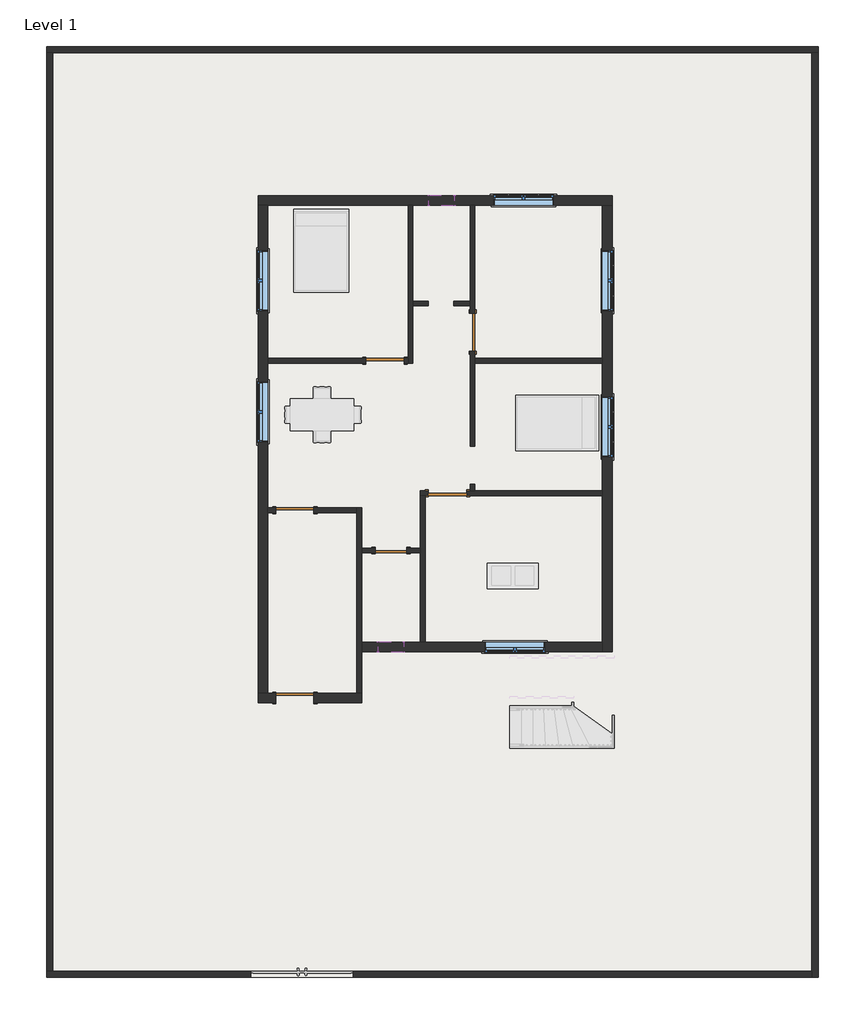
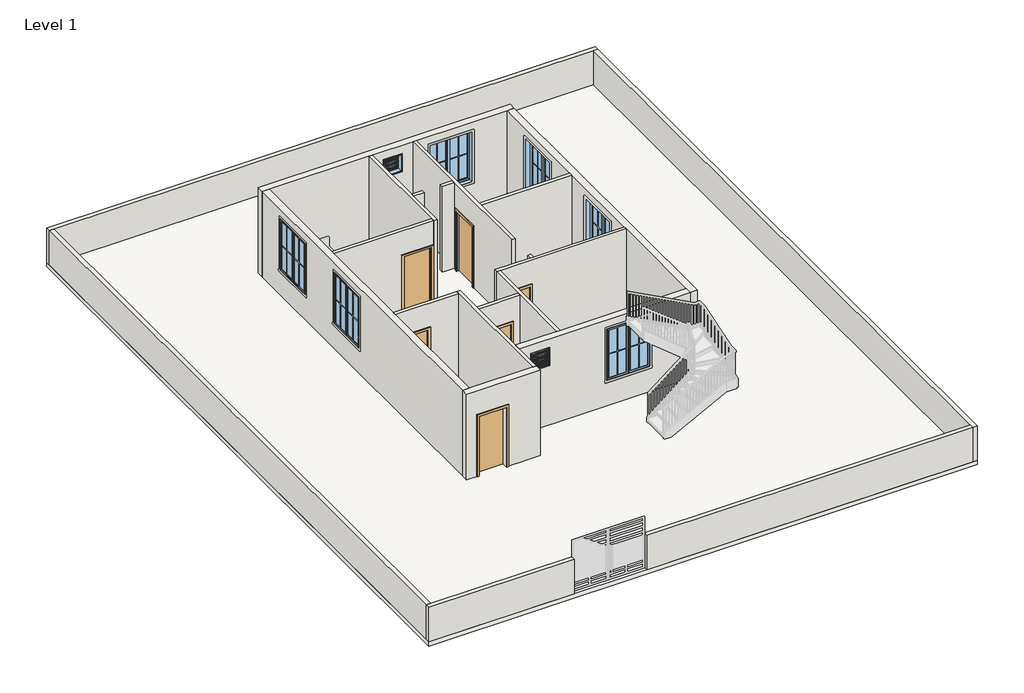
# One storey, part 1 of 3: 22 walls, 8 windows, 6 doors, 1 slab.
"""IFC4 building model written with IfcOpenShell, lengths in millimetres."""

from ifc_helpers import new_model, si_unit, frame, origin, origin_with_axes, place, context, project, spatial, polyline, outline, extrude, faceted_brep, transform, mapped, element, save
from components import door_214872d5, single_flush_door_3_e5f9f3c4, single_flush_door_3_305aa2a5, single_flush_door_3_a90ba1ad, window_9ac97e1a, window_f2d8fef0

model = new_model("IFC4")

# Units and contexts
model_context = context("Model", 3, world=origin())
ifc_project = project(units=[si_unit("LENGTHUNIT", "METRE", prefix="MILLI")], contexts=[model_context])

# Site, building, storey
site = spatial("IfcSite", under=ifc_project)
building = spatial("IfcBuilding", under=site)
storey = spatial("IfcBuildingStorey", under=building, Name="Level 1", Elevation=0.0)

# Doors
placement = place(None, origin())
door_shape = door_214872d5(model_context)
element("IfcDoor", 1, ObjectType="Single-Flush : DOOR 2'6\"", at=placement, inside=storey, context=model_context, shape_type="MappedRepresentation", body=[
    mapped(door_shape, transform((-2309.3144966, -2885.2590409, 0.0), x_axis=(-1.0, 0.0, 0.0), y_axis=(0.0, -1.0, 0.0), z_axis=(0.0, 0.0, 1.0))),
])
single_flush_door_3_shape = single_flush_door_3_e5f9f3c4(model_context)
element("IfcDoor", 2, ObjectType="Single-Flush : DOOR 3'", at=placement, inside=storey, context=model_context, shape_type="MappedRepresentation", body=[
    mapped(single_flush_door_3_shape, transform((-2455.3644966, 1648.6409591, 0.0), x_axis=(1.0, 0.0, 0.0), y_axis=(0.0, 1.0, 0.0), z_axis=(0.0, 0.0, 1.0))),
])
element("IfcDoor", 3, ObjectType="Single-Flush : DOOR 3'", at=placement, inside=storey, context=model_context, shape_type="MappedRepresentation", body=[
    mapped(single_flush_door_3_shape, transform((-359.8644966, 2334.4409591, 0.0), x_axis=(0.0, -1.0, 0.0), y_axis=(1.0, 0.0, 0.0), z_axis=(0.0, 0.0, 1.0))),
])
element("IfcDoor", 4, ObjectType="Single-Flush : DOOR 3'", at=placement, inside=storey, context=model_context, shape_type="MappedRepresentation", body=[
    mapped(single_flush_door_3_shape, transform((-956.7644966, -1513.6590409, 0.0), x_axis=(-1.0, 0.0, 0.0), y_axis=(0.0, -1.0, 0.0), z_axis=(0.0, 0.0, 1.0))),
])
single_flush_door_3_2_shape = single_flush_door_3_305aa2a5(model_context)
element("IfcDoor", 5, ObjectType="Single-Flush : DOOR 3'", at=placement, inside=storey, context=model_context, shape_type="MappedRepresentation", body=[
    mapped(single_flush_door_3_2_shape, transform((-4608.0144966, -1920.0590409, 0.0), x_axis=(-1.0, 0.0, 0.0), y_axis=(0.0, -1.0, 0.0), z_axis=(0.0, 0.0, 1.0))),
])
single_flush_door_3_3_shape = single_flush_door_3_a90ba1ad(model_context)
element("IfcDoor", 6, ObjectType="Single-Flush : DOOR 3'", at=placement, inside=storey, context=model_context, shape_type="MappedRepresentation", body=[
    mapped(single_flush_door_3_3_shape, transform((-4608.0144966, -6409.5090409, 0.0), x_axis=(-1.0, 0.0, 0.0), y_axis=(0.0, -1.0, 0.0), z_axis=(0.0, 0.0, 1.0))),
])

# Slab
element("IfcSlab", 7, ObjectType="FLOOR 6\"", at=placement, inside=storey, context=model_context, shape_type="SweptSolid", body=[
    extrude(outline(polyline([(7897.8751323, 9160.4523528), (7897.8751323, -13089.9476472), (-10542.5248677, -13089.9476472), (-10542.5248677, 9160.4523528), (7897.8751323, 9160.4523528)])), frame((0.0, 0.0, -152.4), z_axis=(0.0, 0.0, 1.0), x_axis=(1.0, 0.0, 0.0)), (0.0, 0.0, 1.0), 152.4),
])

# Walls
element("IfcWall", 8, ObjectType="CMD 6\"", at=placement, inside=storey, context=model_context, shape_type="Brep", body=[
    faceted_brep([(-10542.5248677, 9008.0523528, 0.0), (-10390.1248677, 9008.0523528, 0.0), (7745.4751323, 9008.0523528, 0.0), (7897.8751323, 9008.0523528, 0.0), (7897.8751323, 9008.0523528, 1219.2), (7745.4751323, 9008.0523528, 1219.2), (-10390.1248677, 9008.0523528, 1219.2), (-10542.5248677, 9008.0523528, 1219.2), (-10542.5248677, 9160.4523528, 0.0), (-10542.5248677, 9160.4523528, 1219.2), (7897.8751323, 9160.4523528, 1219.2), (7897.8751323, 9160.4523528, 0.0)], [[[0, 1, 2, 3, 4, 5, 6, 7]], [[8, 9, 10, 11]], [[3, 2, 1, 0, 8, 11]], [[7, 6, 5, 4, 10, 9]], [[4, 3, 11, 10]], [[0, 7, 9, 8]]]),
])
element("IfcWall", 9, ObjectType="CMD 6\"", at=placement, inside=storey, context=model_context, shape_type="Brep", body=[
    faceted_brep([(7745.4751323, 9008.0523528, 0.0), (7745.4751323, -12937.5476472, 0.0), (7745.4751323, -13089.9476472, 0.0), (7745.4751323, -13089.9476472, 1219.2), (7745.4751323, -12937.5476472, 1219.2), (7745.4751323, 9008.0523528, 1219.2), (7897.8751323, 9008.0523528, 0.0), (7897.8751323, 9008.0523528, 1219.2), (7897.8751323, -13089.9476472, 1219.2), (7897.8751323, -13089.9476472, 0.0)], [[[0, 1, 2, 3, 4, 5]], [[6, 7, 8, 9]], [[2, 1, 0, 6, 9]], [[5, 4, 3, 8, 7]], [[0, 5, 7, 6]], [[3, 2, 9, 8]]]),
])
element("IfcWall", 10, ObjectType="CMD 6\"", at=placement, inside=storey, context=model_context, shape_type="SweptSolid", body=[
    extrude(outline(polyline([(-3217.3644966, -12937.5476472), (7745.4751323, -12937.5476472), (7745.4751323, -13089.9476472), (-3217.3644966, -13089.9476472), (-3217.3644966, -12937.5476472)])), origin_with_axes(), (0.0, 0.0, 1.0), 1219.2),
])
element("IfcWall", 11, ObjectType="CMD 6\"", at=placement, inside=storey, context=model_context, shape_type="SweptSolid", body=[
    extrude(outline(polyline([(-10390.1248677, 9008.0523528), (-10390.1248677, -12937.5476472), (-10542.5248677, -12937.5476472), (-10542.5248677, 9008.0523528), (-10390.1248677, 9008.0523528)])), origin_with_axes(), (0.0, 0.0, 1.0), 1219.2),
])
element("IfcWall", 12, ObjectType="CMD 6\"", at=placement, inside=storey, context=model_context, shape_type="Brep", body=[
    faceted_brep([(-5655.7644966, -12937.5476472, 0.0), (-10390.1248677, -12937.5476472, 0.0), (-10542.5248677, -12937.5476472, 0.0), (-10542.5248677, -12937.5476472, 1219.2), (-10390.1248677, -12937.5476472, 1219.2), (-5655.7644966, -12937.5476472, 1219.2), (-5655.7644966, -13089.9476472, 0.0), (-5655.7644966, -13089.9476472, 1219.2), (-10542.5248677, -13089.9476472, 1219.2), (-10542.5248677, -13089.9476472, 0.0)], [[[0, 1, 2, 3, 4, 5]], [[6, 7, 8, 9]], [[2, 1, 0, 6, 9]], [[5, 4, 3, 8, 7]], [[0, 5, 7, 6]], [[3, 2, 9, 8]]]),
])
element("IfcWall", 13, ObjectType="WALL 4.5\"", at=placement, inside=storey, context=model_context, shape_type="Brep", body=[
    faceted_brep([(-1902.9144966, 5363.3909591, 0.0), (-1902.9144966, 1705.7909591, 0.0), (-1902.9144966, 1591.4909591, 0.0), (-1902.9144966, 1591.4909591, 3048.0), (-1902.9144966, 1705.7909591, 3048.0), (-1902.9144966, 5363.3909591, 3048.0), (-1788.6144966, 5363.3909591, 0.0), (-1788.6144966, 5363.3909591, 3048.0), (-1788.6144966, 3077.3909591, 3048.0), (-1788.6144966, 2963.0909591, 3048.0), (-1788.6144966, 1591.4909591, 3048.0), (-1788.6144966, 1591.4909591, 0.0), (-1788.6144966, 2963.0909591, 0.0), (-1788.6144966, 3077.3909591, 0.0)], [[[0, 1, 2, 3, 4, 5]], [[6, 7, 8, 9, 10, 11, 12, 13]], [[2, 1, 0, 6, 13, 12, 11]], [[0, 5, 7, 6]], [[3, 2, 11, 10]], [[5, 4, 3, 10, 9, 8, 7]]]),
])
element("IfcWall", 14, ObjectType="WALL 4.5\"", at=placement, inside=storey, context=model_context, shape_type="SweptSolid", body=[
    extrude(outline(polyline([(2133.6, -1998.1644966), (0.0, -1998.1644966), (0.0, -1902.9144966), (3048.0, -1902.9144966), (3048.0, -5255.7144966), (0.0, -5255.7144966), (0.0, -2912.5644966), (2133.6, -2912.5644966), (2133.6, -1998.1644966)])), frame((0.0, 1591.4909591, 0.0), z_axis=(0.0, 1.0, 0.0), x_axis=(0.0, 0.0, 1.0)), (0.0, 0.0, 1.0), 114.3),
])
element("IfcWall", 15, ObjectType="WALL 4.5\"", at=placement, inside=storey, context=model_context, shape_type="Brep", body=[
    faceted_brep([(-417.0144966, 1877.2409591, 2133.6), (-417.0144966, 1877.2409591, 0.0), (-417.0144966, -389.7090409, 0.0), (-417.0144966, -389.7090409, 3048.0), (-417.0144966, 2963.0909591, 3048.0), (-417.0144966, 3077.3909591, 3048.0), (-417.0144966, 5363.3909591, 3048.0), (-417.0144966, 5363.3909591, 0.0), (-417.0144966, 3077.3909591, 0.0), (-417.0144966, 2963.0909591, 0.0), (-417.0144966, 2791.6409591, 0.0), (-417.0144966, 2791.6409591, 2133.6), (-302.7144966, -389.7090409, 0.0), (-302.7144966, 1591.4909591, 0.0), (-302.7144966, 1705.7909591, 0.0), (-302.7144966, 1877.2409591, 0.0), (-302.7144966, 1877.2409591, 2133.6), (-302.7144966, 2791.6409591, 2133.6), (-302.7144966, 2791.6409591, 0.0), (-302.7144966, 5363.3909591, 0.0), (-302.7144966, 5363.3909591, 3048.0), (-302.7144966, 1705.7909591, 3048.0), (-302.7144966, 1591.4909591, 3048.0), (-302.7144966, -389.7090409, 3048.0)], [[[0, 1, 2, 3, 4, 5, 6, 7, 8, 9, 10, 11]], [[12, 13, 14, 15, 16, 17, 18, 19, 20, 21, 22, 23]], [[2, 1, 15, 14, 13, 12]], [[10, 9, 8, 7, 19, 18]], [[3, 2, 12, 23]], [[7, 6, 20, 19]], [[16, 15, 1, 0]], [[17, 16, 0, 11]], [[18, 17, 11, 10]], [[6, 5, 4, 3, 23, 22, 21, 20]]]),
])
element("IfcWall", 16, ObjectType="WALL 4.5\"", at=placement, inside=storey, context=model_context, shape_type="SweptSolid", body=[
    extrude(outline(polyline([(-302.7144966, 1705.7909591), (2745.2855034, 1705.7909591), (2745.2855034, 1591.4909591), (-302.7144966, 1591.4909591), (-302.7144966, 1705.7909591)])), origin_with_axes(), (0.0, 0.0, 1.0), 3048.0),
])
element("IfcWall", 17, ObjectType="WALL 4.5\"", at=placement, inside=storey, context=model_context, shape_type="SweptSolid", body=[
    extrude(outline(polyline([(-1423.1234474, 2963.0909591), (-1788.6144966, 2963.0909591), (-1788.6144966, 3077.3909591), (-1423.1234474, 3077.3909591), (-1423.1234474, 2963.0909591)])), origin_with_axes(), (0.0, 0.0, 1.0), 3048.0),
])
element("IfcWall", 18, ObjectType="WALL 4.5\"", at=placement, inside=storey, context=model_context, shape_type="Brep", body=[
    faceted_brep([(-1413.9644966, -1456.5090409, 2133.6), (-1413.9644966, -1456.5090409, 0.0), (-1610.8144966, -1456.5090409, 0.0), (-1610.8144966, -1456.5090409, 3048.0), (-417.0144966, -1456.5090409, 3048.0), (-302.7144966, -1456.5090409, 3048.0), (2745.2855034, -1456.5090409, 3048.0), (2745.2855034, -1456.5090409, 0.0), (-302.7144966, -1456.5090409, 0.0), (-417.0144966, -1456.5090409, 0.0), (-499.5644966, -1456.5090409, 0.0), (-499.5644966, -1456.5090409, 2133.6), (-1610.8144966, -1570.8090409, 0.0), (-1496.5144966, -1570.8090409, 0.0), (-1413.9644966, -1570.8090409, 0.0), (-1413.9644966, -1570.8090409, 2133.6), (-499.5644966, -1570.8090409, 2133.6), (-499.5644966, -1570.8090409, 0.0), (2745.2855034, -1570.8090409, 0.0), (2745.2855034, -1570.8090409, 3048.0), (-1496.5144966, -1570.8090409, 3048.0), (-1610.8144966, -1570.8090409, 3048.0)], [[[0, 1, 2, 3, 4, 5, 6, 7, 8, 9, 10, 11]], [[12, 13, 14, 15, 16, 17, 18, 19, 20, 21]], [[2, 1, 14, 13, 12]], [[10, 9, 8, 7, 18, 17]], [[7, 6, 19, 18]], [[3, 2, 12, 21]], [[15, 14, 1, 0]], [[16, 15, 0, 11]], [[17, 16, 11, 10]], [[6, 5, 4, 3, 21, 20, 19]]]),
])
element("IfcWall", 19, ObjectType="WALL 4.5\"", at=placement, inside=storey, context=model_context, shape_type="SweptSolid", body=[
    extrude(outline(polyline([(-302.7144966, -1304.1090409), (-302.7144966, -1456.5090409), (-417.0144966, -1456.5090409), (-417.0144966, -1304.1090409), (-302.7144966, -1304.1090409)])), origin_with_axes(), (0.0, 0.0, 1.0), 3048.0),
])
element("IfcWall", 20, ObjectType="WALL 4.5\"", at=placement, inside=storey, context=model_context, shape_type="Brep", body=[
    faceted_brep([(-1610.8144966, -1570.8090409, 0.0), (-1610.8144966, -2828.1090409, 0.0), (-1610.8144966, -2942.4090409, 0.0), (-1610.8144966, -5076.0090409, 0.0), (-1610.8144966, -5076.0090409, 3048.0), (-1610.8144966, -2942.4090409, 3048.0), (-1610.8144966, -2828.1090409, 3048.0), (-1610.8144966, -1570.8090409, 3048.0), (-1496.5144966, -1570.8090409, 0.0), (-1496.5144966, -1570.8090409, 3048.0), (-1496.5144966, -5076.0090409, 3048.0), (-1496.5144966, -5076.0090409, 0.0)], [[[0, 1, 2, 3, 4, 5, 6, 7]], [[8, 9, 10, 11]], [[3, 2, 1, 0, 8, 11]], [[0, 7, 9, 8]], [[4, 3, 11, 10]], [[7, 6, 5, 4, 10, 9]]]),
])
element("IfcWall", 21, ObjectType="WALL 4.5\"", at=placement, inside=storey, context=model_context, shape_type="SweptSolid", body=[
    extrude(outline(polyline([(0.0, -3007.8144966), (0.0, -2690.3144966), (2133.6, -2690.3144966), (2133.6, -1928.3144966), (0.0, -1928.3144966), (0.0, -1610.8144966), (3048.0, -1610.8144966), (3048.0, -3007.8144966), (0.0, -3007.8144966)])), frame((0.0, -2942.4090409, 0.0), z_axis=(0.0, 1.0, 0.0), x_axis=(0.0, 0.0, 1.0)), (0.0, 0.0, 1.0), 114.3),
])
element("IfcWall", 22, ObjectType="WALL 4.5\"", at=placement, inside=storey, context=model_context, shape_type="Brep", body=[
    faceted_brep([(-3007.8144966, -6295.2090409, 0.0), (-3007.8144966, -5304.6090409, 0.0), (-3007.8144966, -5076.0090409, 0.0), (-3007.8144966, -2942.4090409, 0.0), (-3007.8144966, -2828.1090409, 0.0), (-3007.8144966, -1862.9090409, 0.0), (-3007.8144966, -1862.9090409, 3048.0), (-3007.8144966, -2828.1090409, 3048.0), (-3007.8144966, -2942.4090409, 3048.0), (-3007.8144966, -5076.0090409, 3048.0), (-3007.8144966, -5304.6090409, 3048.0), (-3007.8144966, -6295.2090409, 3048.0), (-3122.1144966, -6295.2090409, 0.0), (-3122.1144966, -6295.2090409, 3048.0), (-3122.1144966, -1977.2090409, 3048.0), (-3122.1144966, -1862.9090409, 3048.0), (-3122.1144966, -1862.9090409, 0.0), (-3122.1144966, -1977.2090409, 0.0)], [[[0, 1, 2, 3, 4, 5, 6, 7, 8, 9, 10, 11]], [[12, 13, 14, 15, 16, 17]], [[5, 4, 3, 2, 1, 0, 12, 17, 16]], [[0, 11, 13, 12]], [[6, 5, 16, 15]], [[11, 10, 9, 8, 7, 6, 15, 14, 13]]]),
])
element("IfcWall", 23, ObjectType="WALL 4.5\"", at=placement, inside=storey, context=model_context, shape_type="SweptSolid", body=[
    extrude(outline(polyline([(0.0, -5255.7144966), (0.0, -5065.2144966), (2133.6, -5065.2144966), (2133.6, -4150.8144966), (0.0, -4150.8144966), (0.0, -3122.1144966), (3048.0, -3122.1144966), (3048.0, -5255.7144966), (0.0, -5255.7144966)])), frame((0.0, -1977.2090409, 0.0), z_axis=(0.0, 1.0, 0.0), x_axis=(0.0, 0.0, 1.0)), (0.0, 0.0, 1.0), 114.3),
])
element("IfcWall", 24, ObjectType="WALL 4.5\"", at=placement, inside=storey, context=model_context, shape_type="SweptSolid", body=[
    extrude(outline(polyline([(-417.0144966, 2963.0909591), (-814.3659123, 2963.0909591), (-814.3659123, 3077.3909591), (-417.0144966, 3077.3909591), (-417.0144966, 2963.0909591)])), origin_with_axes(), (0.0, 0.0, 1.0), 3048.0),
])
element("IfcWall", 25, ObjectType="WALL 9\"", at=placement, inside=storey, context=model_context, shape_type="Brep", body=[
    faceted_brep([(-5484.3144966, 5363.3909591, 0.0), (-5255.7144966, 5363.3909591, 0.0), (-1902.9144966, 5363.3909591, 0.0), (-1788.6144966, 5363.3909591, 0.0), (-417.0144966, 5363.3909591, 0.0), (-302.7144966, 5363.3909591, 0.0), (2745.2855034, 5363.3909591, 0.0), (2973.8855034, 5363.3909591, 0.0), (2973.8855034, 5363.3909591, 3048.0), (2745.2855034, 5363.3909591, 3048.0), (-302.7144966, 5363.3909591, 3048.0), (-417.0144966, 5363.3909591, 3048.0), (-1788.6144966, 5363.3909591, 3048.0), (-1902.9144966, 5363.3909591, 3048.0), (-5255.7144966, 5363.3909591, 3048.0), (-5484.3144966, 5363.3909591, 3048.0), (1583.2355034, 5363.3909591, 2743.2), (1583.2355034, 5363.3909591, 914.4), (135.4355034, 5363.3909591, 914.4), (135.4355034, 5363.3909591, 2743.2), (-1407.6144966, 5363.3909591, 2743.2), (-798.0144966, 5363.3909591, 2743.2), (-798.0144966, 5363.3909591, 2133.6), (-1407.6144966, 5363.3909591, 2133.6), (-5484.3144966, 5591.9909591, 0.0), (-5484.3144966, 5591.9909591, 3048.0), (2973.8855034, 5591.9909591, 3048.0), (2973.8855034, 5591.9909591, 0.0), (1583.2355034, 5591.9909591, 2743.2), (135.4355034, 5591.9909591, 2743.2), (135.4355034, 5591.9909591, 914.4), (1583.2355034, 5591.9909591, 914.4), (-1407.6144966, 5591.9909591, 2743.2), (-1407.6144966, 5591.9909591, 2133.6), (-798.0144966, 5591.9909591, 2133.6), (-798.0144966, 5591.9909591, 2743.2)], [[[0, 1, 2, 3, 4, 5, 6, 7, 8, 9, 10, 11, 12, 13, 14, 15], [16, 17, 18, 19], [20, 21, 22, 23]], [[24, 25, 26, 27], [28, 29, 30, 31], [32, 33, 34, 35]], [[7, 6, 5, 4, 3, 2, 1, 0, 24, 27]], [[8, 7, 27, 26]], [[0, 15, 25, 24]], [[17, 16, 28, 31]], [[18, 17, 31, 30]], [[19, 18, 30, 29]], [[16, 19, 29, 28]], [[33, 32, 20, 23]], [[34, 33, 23, 22]], [[35, 34, 22, 21]], [[32, 35, 21, 20]], [[15, 14, 13, 12, 11, 10, 9, 8, 26, 25]]]),
])
element("IfcWall", 26, ObjectType="WALL 9\"", at=placement, inside=storey, context=model_context, shape_type="Brep", body=[
    faceted_brep([(2745.2855034, 5363.3909591, 0.0), (2745.2855034, 1705.7909591, 0.0), (2745.2855034, 1591.4909591, 0.0), (2745.2855034, -1456.5090409, 0.0), (2745.2855034, -1570.8090409, 0.0), (2745.2855034, -5076.0090409, 0.0), (2745.2855034, -5304.6090409, 0.0), (2745.2855034, -5304.6090409, 3048.0), (2745.2855034, -5076.0090409, 3048.0), (2745.2855034, -1570.8090409, 3048.0), (2745.2855034, -1456.5090409, 3048.0), (2745.2855034, 1591.4909591, 3048.0), (2745.2855034, 1705.7909591, 3048.0), (2745.2855034, 5363.3909591, 3048.0), (2745.2855034, -656.4090409, 2743.2), (2745.2855034, -656.4090409, 914.4), (2745.2855034, 791.3909591, 914.4), (2745.2855034, 791.3909591, 2743.2), (2745.2855034, 2839.2659591, 2743.2), (2745.2855034, 2839.2659591, 914.4), (2745.2855034, 4287.0659591, 914.4), (2745.2855034, 4287.0659591, 2743.2), (2973.8855034, 5363.3909591, 0.0), (2973.8855034, 5363.3909591, 3048.0), (2973.8855034, -5304.6090409, 3048.0), (2973.8855034, -5304.6090409, 0.0), (2973.8855034, -656.4090409, 2743.2), (2973.8855034, 791.3909591, 2743.2), (2973.8855034, 791.3909591, 914.4), (2973.8855034, -656.4090409, 914.4), (2973.8855034, 2839.2659591, 2743.2), (2973.8855034, 4287.0659591, 2743.2), (2973.8855034, 4287.0659591, 914.4), (2973.8855034, 2839.2659591, 914.4)], [[[0, 1, 2, 3, 4, 5, 6, 7, 8, 9, 10, 11, 12, 13], [14, 15, 16, 17], [18, 19, 20, 21]], [[22, 23, 24, 25], [26, 27, 28, 29], [30, 31, 32, 33]], [[6, 5, 4, 3, 2, 1, 0, 22, 25]], [[0, 13, 23, 22]], [[7, 6, 25, 24]], [[15, 14, 26, 29]], [[16, 15, 29, 28]], [[17, 16, 28, 27]], [[14, 17, 27, 26]], [[19, 18, 30, 33]], [[20, 19, 33, 32]], [[21, 20, 32, 31]], [[18, 21, 31, 30]], [[13, 12, 11, 10, 9, 8, 7, 24, 23]]]),
])
element("IfcWall", 27, ObjectType="WALL 9\"", at=placement, inside=storey, context=model_context, shape_type="Brep", body=[
    faceted_brep([(2745.2855034, -5076.0090409, 0.0), (-1496.5144966, -5076.0090409, 0.0), (-1610.8144966, -5076.0090409, 0.0), (-3007.8144966, -5076.0090409, 0.0), (-3007.8144966, -5076.0090409, 3048.0), (-1610.8144966, -5076.0090409, 3048.0), (-1496.5144966, -5076.0090409, 3048.0), (2745.2855034, -5076.0090409, 3048.0), (-70.9394966, -5076.0090409, 2743.2), (-70.9394966, -5076.0090409, 914.4), (1376.8605034, -5076.0090409, 914.4), (1376.8605034, -5076.0090409, 2743.2), (-2004.5144966, -5076.0090409, 2743.2), (-2614.1144966, -5076.0090409, 2743.2), (-2614.1144966, -5076.0090409, 2133.6), (-2004.5144966, -5076.0090409, 2133.6), (2745.2855034, -5304.6090409, 0.0), (2745.2855034, -5304.6090409, 3048.0), (-3007.8144966, -5304.6090409, 3048.0), (-3007.8144966, -5304.6090409, 0.0), (-70.9394966, -5304.6090409, 2743.2), (1376.8605034, -5304.6090409, 2743.2), (1376.8605034, -5304.6090409, 914.4), (-70.9394966, -5304.6090409, 914.4), (-2004.5144966, -5304.6090409, 2743.2), (-2004.5144966, -5304.6090409, 2133.6), (-2614.1144966, -5304.6090409, 2133.6), (-2614.1144966, -5304.6090409, 2743.2)], [[[0, 1, 2, 3, 4, 5, 6, 7], [8, 9, 10, 11], [12, 13, 14, 15]], [[16, 17, 18, 19], [20, 21, 22, 23], [24, 25, 26, 27]], [[3, 2, 1, 0, 16, 19]], [[0, 7, 17, 16]], [[4, 3, 19, 18]], [[9, 8, 20, 23]], [[10, 9, 23, 22]], [[11, 10, 22, 21]], [[8, 11, 21, 20]], [[25, 24, 12, 15]], [[26, 25, 15, 14]], [[27, 26, 14, 13]], [[24, 27, 13, 12]], [[7, 6, 5, 4, 18, 17]]]),
])
element("IfcWall", 28, ObjectType="WALL 9\"", at=placement, inside=storey, context=model_context, shape_type="Brep", body=[
    faceted_brep([(-5065.2144966, -6295.2090409, 2133.6), (-5065.2144966, -6295.2090409, 0.0), (-5255.7144966, -6295.2090409, 0.0), (-5484.3144966, -6295.2090409, 0.0), (-5484.3144966, -6295.2090409, 3048.0), (-5255.7144966, -6295.2090409, 3048.0), (-3122.1144966, -6295.2090409, 3048.0), (-3007.8144966, -6295.2090409, 3048.0), (-3007.8144966, -6295.2090409, 0.0), (-3122.1144966, -6295.2090409, 0.0), (-4150.8144966, -6295.2090409, 0.0), (-4150.8144966, -6295.2090409, 2133.6), (-5484.3144966, -6523.8090409, 0.0), (-5065.2144966, -6523.8090409, 0.0), (-5065.2144966, -6523.8090409, 2133.6), (-4150.8144966, -6523.8090409, 2133.6), (-4150.8144966, -6523.8090409, 0.0), (-3007.8144966, -6523.8090409, 0.0), (-3007.8144966, -6523.8090409, 3048.0), (-5484.3144966, -6523.8090409, 3048.0)], [[[0, 1, 2, 3, 4, 5, 6, 7, 8, 9, 10, 11]], [[12, 13, 14, 15, 16, 17, 18, 19]], [[10, 9, 8, 17, 16]], [[3, 2, 1, 13, 12]], [[4, 3, 12, 19]], [[8, 7, 18, 17]], [[7, 6, 5, 4, 19, 18]], [[14, 13, 1, 0]], [[15, 14, 0, 11]], [[16, 15, 11, 10]]]),
])
element("IfcWall", 29, ObjectType="WALL 9\"", at=placement, inside=storey, context=model_context, shape_type="Brep", body=[
    faceted_brep([(-5255.7144966, -6295.2090409, 0.0), (-5255.7144966, -1977.2090409, 0.0), (-5255.7144966, -1862.9090409, 0.0), (-5255.7144966, 1591.4909591, 0.0), (-5255.7144966, 1705.7909591, 0.0), (-5255.7144966, 5363.3909591, 0.0), (-5255.7144966, 5363.3909591, 3048.0), (-5255.7144966, 1705.7909591, 3048.0), (-5255.7144966, 1591.4909591, 3048.0), (-5255.7144966, -1862.9090409, 3048.0), (-5255.7144966, -1977.2090409, 3048.0), (-5255.7144966, -6295.2090409, 3048.0), (-5255.7144966, 4287.0659591, 2743.2), (-5255.7144966, 4287.0659591, 914.4), (-5255.7144966, 2839.2659591, 914.4), (-5255.7144966, 2839.2659591, 2743.2), (-5255.7144966, 1153.3409591, 2743.2), (-5255.7144966, 1153.3409591, 914.4), (-5255.7144966, -294.4590409, 914.4), (-5255.7144966, -294.4590409, 2743.2), (-5484.3144966, -6295.2090409, 0.0), (-5484.3144966, -6295.2090409, 3048.0), (-5484.3144966, 5363.3909591, 3048.0), (-5484.3144966, 5363.3909591, 0.0), (-5484.3144966, 4287.0659591, 2743.2), (-5484.3144966, 2839.2659591, 2743.2), (-5484.3144966, 2839.2659591, 914.4), (-5484.3144966, 4287.0659591, 914.4), (-5484.3144966, 1153.3409591, 2743.2), (-5484.3144966, -294.4590409, 2743.2), (-5484.3144966, -294.4590409, 914.4), (-5484.3144966, 1153.3409591, 914.4)], [[[0, 1, 2, 3, 4, 5, 6, 7, 8, 9, 10, 11], [12, 13, 14, 15], [16, 17, 18, 19]], [[20, 21, 22, 23], [24, 25, 26, 27], [28, 29, 30, 31]], [[5, 4, 3, 2, 1, 0, 20, 23]], [[0, 11, 21, 20]], [[6, 5, 23, 22]], [[13, 12, 24, 27]], [[14, 13, 27, 26]], [[15, 14, 26, 25]], [[12, 15, 25, 24]], [[17, 16, 28, 31]], [[18, 17, 31, 30]], [[19, 18, 30, 29]], [[16, 19, 29, 28]], [[11, 10, 9, 8, 7, 6, 22, 21]]]),
])

# Windows
window_shape = window_9ac97e1a(model_context)
element("IfcWindow", 30, ObjectType="Window-Casement-Double : 57\" x 72\"", at=placement, inside=storey, context=model_context, shape_type="MappedRepresentation", body=[
    mapped(window_shape, transform((2859.5855034, 67.4909591, 0.0), x_axis=(0.0, -1.0, 0.0), y_axis=(1.0, 0.0, 0.0), z_axis=(0.0, 0.0, 1.0))),
])
element("IfcWindow", 31, ObjectType="Window-Casement-Double : 57\" x 72\"", at=placement, inside=storey, context=model_context, shape_type="MappedRepresentation", body=[
    mapped(window_shape, transform((2859.5855034, 3563.1659591, 0.0), x_axis=(0.0, -1.0, 0.0), y_axis=(1.0, 0.0, 0.0), z_axis=(0.0, 0.0, 1.0))),
])
element("IfcWindow", 32, ObjectType="Window-Casement-Double : 57\" x 72\"", at=placement, inside=storey, context=model_context, shape_type="MappedRepresentation", body=[
    mapped(window_shape, transform((859.3355034, 5477.6909591, 0.0), x_axis=(1.0, 0.0, 0.0), y_axis=(0.0, 1.0, 0.0), z_axis=(0.0, 0.0, 1.0))),
])
element("IfcWindow", 33, ObjectType="Window-Casement-Double : 57\" x 72\"", at=placement, inside=storey, context=model_context, shape_type="MappedRepresentation", body=[
    mapped(window_shape, transform((-5370.0144966, 3563.1659591, 0.0), x_axis=(0.0, 1.0, 0.0), y_axis=(-1.0, 0.0, 0.0), z_axis=(0.0, 0.0, 1.0))),
])
element("IfcWindow", 34, ObjectType="Window-Casement-Double : 57\" x 72\"", at=placement, inside=storey, context=model_context, shape_type="MappedRepresentation", body=[
    mapped(window_shape, transform((-5370.0144966, 429.4409591, 0.0), x_axis=(0.0, 1.0, 0.0), y_axis=(-1.0, 0.0, 0.0), z_axis=(0.0, 0.0, 1.0))),
])
element("IfcWindow", 35, ObjectType="Window-Casement-Double : 57\" x 72\"", at=placement, inside=storey, context=model_context, shape_type="MappedRepresentation", body=[
    mapped(window_shape, transform((652.9605034, -5190.3090409, 0.0), x_axis=(-1.0, 0.0, 0.0), y_axis=(0.0, -1.0, 0.0), z_axis=(0.0, 0.0, 1.0))),
])
window_2_shape = window_f2d8fef0(model_context)
element("IfcWindow", 36, ObjectType="Window-Louvers : 24\" x 24\"", at=placement, inside=storey, context=model_context, shape_type="MappedRepresentation", body=[
    mapped(window_2_shape, transform((-1102.8144966, 5484.0409591, 1219.2), x_axis=(1.0, 0.0, 0.0), y_axis=(0.0, 1.0, 0.0), z_axis=(0.0, 0.0, 1.0))),
])
element("IfcWindow", 37, ObjectType="Window-Louvers : 24\" x 24\"", at=placement, inside=storey, context=model_context, shape_type="MappedRepresentation", body=[
    mapped(window_2_shape, transform((-2309.3144966, -5196.6590409, 1219.2), x_axis=(-1.0, 0.0, 0.0), y_axis=(0.0, -1.0, 0.0), z_axis=(0.0, 0.0, 1.0))),
])

save(model, "model.ifc")

# Revit data of these elements
# Type "Single-Flush : DOOR 2'6\""
#   Type Mark = "10"
#   Construction Type Id = "MDOOR"
#   Assembly Code = "C1020"
#   Analytic Construction = "Metal"
#   Thickness = 0' - 2"
#   Heat Transfer Coefficient (U) = 0.651978 BTU/(h·ft²·°F)
#   Height = 7' - 0"
#   Trim Projection Ext = 0' - 1"
#   Trim Projection Int = 0' - 1"
#   Trim Width = 0' - 3"
#   Width = 2' - 6"
#   Define Thermal Properties by = 1
#   Door Material = Door - Panel
#   Frame Material = Door - Frame
#   Visual Light Transmittance = 0
#   Solar Heat Gain Coefficient = 0
#   Function = (empty or 0)
#   Wall Closure = (empty or 0)
# Type "Single-Flush : DOOR 3'"
#   Type Mark = "9"
#   Construction Type Id = "MDOOR"
#   Assembly Code = "C1020"
#   Analytic Construction = "Metal"
#   Thickness = 0' - 2"
#   Heat Transfer Coefficient (U) = 0.651978 BTU/(h·ft²·°F)
#   Height = 7' - 0"
#   Trim Projection Ext = 0' - 1"
#   Trim Projection Int = 0' - 1"
#   Trim Width = 0' - 3"
#   Width = 3' - 0"
#   Define Thermal Properties by = 1
#   Door Material = Door - Panel
#   Frame Material = Door - Frame
#   Visual Light Transmittance = 0
#   Solar Heat Gain Coefficient = 0
#   Function = (empty or 0)
#   Wall Closure = (empty or 0)
# Type "FLOOR 6\""
#   Assembly Code = "B1010"
#   Function = 0
#   Layers, outside or top first: 0' - 6" no material (function 1)
# Type "CMD 6\""
#   Assembly Code = "B2010"
#   Layers, outside or top first: 0' - 6" no material (function 1)
# Type "WALL 4.5\""
#   Assembly Code = "B2010"
#   Layers, outside or top first: 0' - 4 1/2" no material (function 1)
# Type "WALL 9\""
#   Assembly Code = "B2010"
#   Layers, outside or top first: 0' - 9" no material (function 1)
# Type "Window-Casement-Double : 57\" x 72\""
#   Type Mark = "17"
#   Fire Rating = "0.5h"
#   Assembly Code = "B2020100"
#   Analytic Construction = "Double glazing - domestic"
#   Frame Extension [instance default] = 0' - 0 1/4"
#   Window Inset [instance default] = 0' - 0"
#   Wall Thickness [instance default] = 0' - 6"
#   Interior Wall Closure [instance default] = 0' - 2 1/4"
#   Half Width = 2' - 4 1/2"
#   Visual Light Transmittance = 0.81
#   Thermal Resistance (R) = 1.8146 (h·ft²·°F)/BTU
#   Solar Heat Gain Coefficient = 0.76
#   Rough Width = 4' - 9 1/2"
#   Rough Height = 6' - 0 1/2"
#   Height = 6' - 0"
#   Heat Transfer Coefficient (U) = 0.5511 BTU/(h·ft²·°F)
#   Exterior Wall Closure [instance default] = 0' - 1 1/4"
#   Extension Jamb [instance default] = 0' - 2 1/4"
#   Default Sill Height = 3' - 0"
#   Width = 4' - 9"
#   Define Thermal Properties by = 0
#   Muntin Visibility = yes
#   Interior Trim Visibility [instance default] = yes
#   Exterior Trim Visibility [instance default] = yes
#   Extension Jamb Visibility [instance default] = yes
#   Interior Trim Material = Wood - Stained
#   Muntin Pattern = Muntin Pattern_2x2 : Muntin Pattern_2x2
#   Interior Trim = Trim-Window-Interior-Flat : Picture Frame
#   Interior Frame Material = Wood - Stained
#   Glass Panel Material = Glass
#   Exterior Trim Material = Clad - White
#   Exterior Trim = Trim-Window-Exterior-Flat : with Sill
#   Exterior Frame Material = Clad - White
#   Wall Closure = (empty or 0)
# Type "Window-Louvers : 24\" x 24\""
#   Type Mark = "18"
#   Construction Type Id = "GSP4R"
#   Assembly Code = "B20"
#   Analytic Construction = "1/8 in Pilkington single glazing"
#   Visual Light Transmittance = 0.9
#   Thermal Resistance (R) = 1.53941 (h·ft²·°F)/BTU
#   Solar Heat Gain Coefficient = 0.78
#   Max Height = 1' - 11.74264"
#   Height = 2' - 0"
#   Heat Transfer Coefficient (U) = 0.6496 BTU/(h·ft²·°F)
#   Blade Width [instance default] = 1' - 10 1/2"
#   Blade Vertical Thickness = 0' - 0.35355"
#   Blade Thickness = 0' - 0 1/4"
#   Blade Spacing = 0' - 1 1/2"
#   Blade Height = 0' - 1.85355"
#   Blade Depth = 0' - 3"
#   Blade Angle = 45.00°
#   Default Sill Height = 3' - 0"
#   Trim Projection_Exterior = 0' - 0 1/2"
#   Trim Projection_Interior = 0' - 0 1/2"
#   Trim Width_Exterior = 0' - 1 1/2"
#   Trim Width_Interior = 0' - 1 1/2"
#   Width = 2' - 0"
#   Max Blade Count = 12
#   Define Thermal Properties by = 1
#   Blade Count = 12
#   Frame Material = Birch
#   Louver Material = Birch
#   Trim Exterior Material = Birch
#   Trim Interior Material = Birch
#   Wall Closure = (empty or 0)
# Element 1 (IfcDoor, "Single-Flush : DOOR 2'6\"")
#   Phase Created = New Construction
#   Materials on its faces: "Door - Frame", "Door - Panel"
# Elements 2, 3, 4, 5, 6 (IfcDoor, "Single-Flush : DOOR 3'")
#   Phase Created = New Construction
#   Materials on its faces: "Door - Frame", "Door - Panel"
# Element 7 (IfcSlab, "FLOOR 6\"")
#   Height Offset From Level = 0' - 0"
#   Phase Created = New Construction
#   Materials on its faces: "Cherry", "Default Floor", "Softwood, Lumber"
# Elements 8, 9, 12 (IfcWall, "CMD 6\"")
#   Top Offset = 0' - 0"
#   Base Offset = 0' - 0"
#   Unconnected Height = 4' - 0"
#   wall height = 4' - 0"
#   Phase Created = New Construction
#   Base Constraint = Level 1
#   Materials on its faces: "Clad - White", "Default Wall", "Cherry"
# Elements 10, 11 (IfcWall, "CMD 6\"")
#   Top Offset = 0' - 0"
#   Base Offset = 0' - 0"
#   Unconnected Height = 4' - 0"
#   wall height = 4' - 0"
#   Phase Created = New Construction
#   Base Constraint = Level 1
#   Materials on its faces: "Default Wall", "Clad - White", "Cherry"
# Elements 13, 14, 15, 16, 17, 18, 19, 20, 21, 22, 23, 24 (IfcWall, "WALL 4.5\"")
#   Top Offset = 0' - 0"
#   Base Offset = 0' - 0"
#   Unconnected Height = 10' - 0"
#   wall height = 10' - 0"
#   Phase Created = New Construction
#   Base Constraint = Level 1
#   Materials on its faces: "Default Wall"
# Elements 25, 26, 27, 28, 29 (IfcWall, "WALL 9\"")
#   Top Offset = 0' - 0"
#   Base Offset = 0' - 0"
#   Unconnected Height = 10' - 0"
#   wall height = 10' - 0"
#   Phase Created = New Construction
#   Base Constraint = Level 1
#   Materials on its faces: "Default Wall"
# Element 30 (IfcWindow, "Window-Casement-Double : 57\" x 72\"")
#   Mark = "1"
#   Window Inset = 0' - 0"
#   Interior Wall Closure = 0' - 2 1/4"
#   Frame Extension = 0' - 0 1/4"
#   Exterior Wall Closure = 0' - 1 1/4"
#   Interior Trim Visibility = yes
#   Exterior Trim Visibility = yes
#   Phase Created = New Construction
#   Materials on its faces: "Wood - Stained", "Glass", "Clad - White"
# Element 31 (IfcWindow, "Window-Casement-Double : 57\" x 72\"")
#   Mark = "2"
#   Window Inset = 0' - 0"
#   Interior Wall Closure = 0' - 2 1/4"
#   Frame Extension = 0' - 0 1/4"
#   Exterior Wall Closure = 0' - 1 1/4"
#   Interior Trim Visibility = yes
#   Exterior Trim Visibility = yes
#   Phase Created = New Construction
#   Materials on its faces: "Wood - Stained", "Glass", "Clad - White"
# Element 32 (IfcWindow, "Window-Casement-Double : 57\" x 72\"")
#   Mark = "3"
#   Window Inset = 0' - 0"
#   Interior Wall Closure = 0' - 2 1/4"
#   Frame Extension = 0' - 0 1/4"
#   Exterior Wall Closure = 0' - 1 1/4"
#   Interior Trim Visibility = yes
#   Exterior Trim Visibility = yes
#   Phase Created = New Construction
#   Materials on its faces: "Wood - Stained", "Glass", "Clad - White"
# Element 33 (IfcWindow, "Window-Casement-Double : 57\" x 72\"")
#   Mark = "4"
#   Window Inset = 0' - 0"
#   Interior Wall Closure = 0' - 2 1/4"
#   Frame Extension = 0' - 0 1/4"
#   Exterior Wall Closure = 0' - 1 1/4"
#   Interior Trim Visibility = yes
#   Exterior Trim Visibility = yes
#   Phase Created = New Construction
#   Materials on its faces: "Wood - Stained", "Glass", "Clad - White"
# Element 34 (IfcWindow, "Window-Casement-Double : 57\" x 72\"")
#   Mark = "5"
#   Window Inset = 0' - 0"
#   Interior Wall Closure = 0' - 2 1/4"
#   Frame Extension = 0' - 0 1/4"
#   Exterior Wall Closure = 0' - 1 1/4"
#   Interior Trim Visibility = yes
#   Exterior Trim Visibility = yes
#   Phase Created = New Construction
#   Materials on its faces: "Wood - Stained", "Glass", "Clad - White"
# Element 35 (IfcWindow, "Window-Casement-Double : 57\" x 72\"")
#   Mark = "6"
#   Window Inset = 0' - 0"
#   Interior Wall Closure = 0' - 2 1/4"
#   Frame Extension = 0' - 0 1/4"
#   Exterior Wall Closure = 0' - 1 1/4"
#   Interior Trim Visibility = yes
#   Exterior Trim Visibility = yes
#   Phase Created = New Construction
#   Materials on its faces: "Wood - Stained", "Glass", "Clad - White"
# Element 36 (IfcWindow, "Window-Louvers : 24\" x 24\"")
#   Mark = "7"
#   Blade Width = 1' - 10 1/2"
#   Phase Created = New Construction
#   Materials on its faces: "Birch"
# Element 37 (IfcWindow, "Window-Louvers : 24\" x 24\"")
#   Mark = "8"
#   Blade Width = 1' - 10 1/2"
#   Phase Created = New Construction
#   Materials on its faces: "Birch"
# Materials
#   "Door - Panel": class "Wood", colour RGB 210 159 95, transparency 0, Cost = 0
#   "Door - Frame": colour RGB 118 70 51, transparency 0, Cost = 0
#   "Wood - Stained": class "Wood", colour RGB 224 178 126, transparency 0, Cost = 0
#   "Glass": class "Glass", colour RGB 0 128 192, transparency 0.75, Description = "Soda Lime Glass", Cost = 0
#   "Clad - White": class "Wood", colour RGB 242 242 238, transparency 0, Cost = 0
#   "Birch": class "Wood", colour RGB 224 178 126, transparency 0, Description = "Betula Alleghaniensis", Cost = 0
#   "Cherry": class "Wood", colour RGB 226 177 128, transparency 0, Description = "Prunus Serotina", Cost = 0
#   "Default Floor": colour RGB 128 128 128, transparency 0, Cost = 0
#   "Softwood, Lumber": class "Wood", colour RGB 223 192 134, transparency 0, Description = "Pinus Echinata", Cost = 0
#   "Default Wall": colour RGB 128 128 128, transparency 0, Cost = 0
